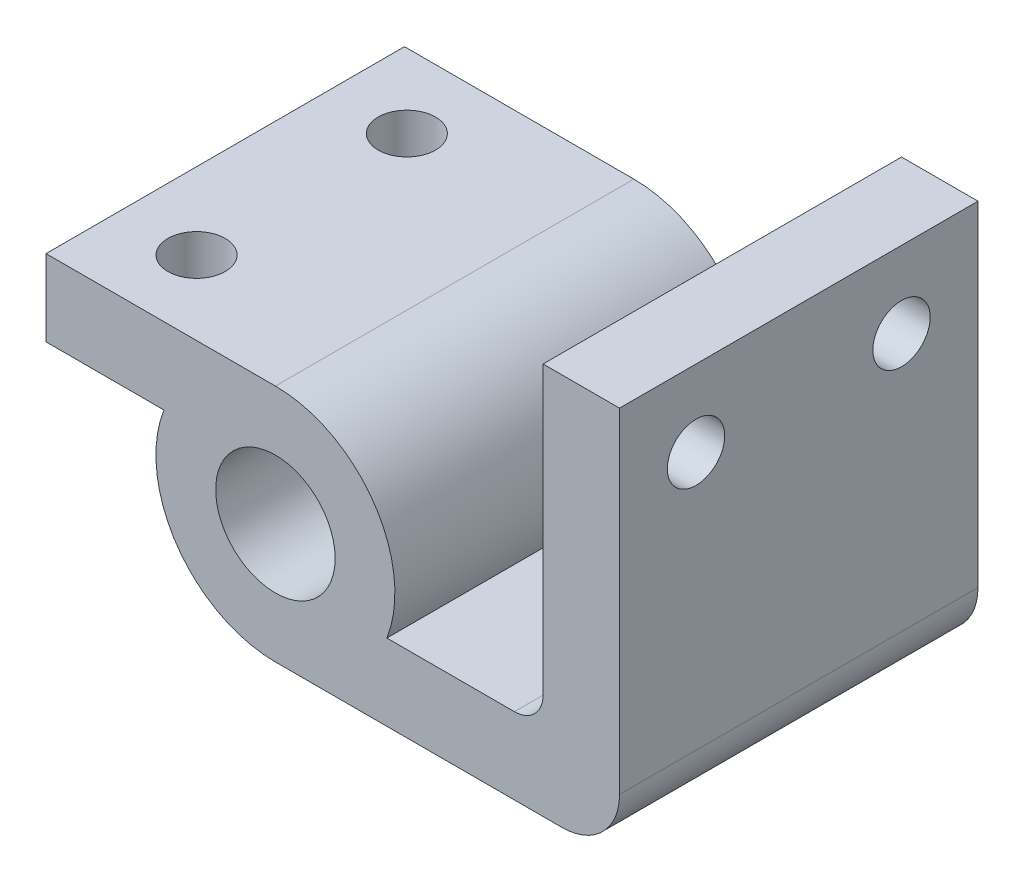
ISO-10303-21;
HEADER;
FILE_DESCRIPTION(('STEP AP214'),'2;1');
FILE_NAME('part.step','',(''),(''),'','','');
FILE_SCHEMA(('AUTOMOTIVE_DESIGN { 1 0 10303 214 1 1 1 1 }'));
ENDSEC;
DATA;
#1=APPLICATION_CONTEXT('core data for automotive mechanical design processes');
#2=APPLICATION_PROTOCOL_DEFINITION('international standard','automotive_design',2000,#1);
#3=PRODUCT_CONTEXT('',#1,'mechanical');
#4=PRODUCT('Part','Part','',(#3));
#5=PRODUCT_RELATED_PRODUCT_CATEGORY('part','',(#4));
#6=PRODUCT_DEFINITION_FORMATION('','',#4);
#7=PRODUCT_DEFINITION_CONTEXT('part definition',#1,'design');
#8=PRODUCT_DEFINITION('design','',#6,#7);
#9=PRODUCT_DEFINITION_SHAPE('','',#8);
#10=(LENGTH_UNIT() NAMED_UNIT(*) SI_UNIT(.MILLI.,.METRE.));
#11=(NAMED_UNIT(*) PLANE_ANGLE_UNIT() SI_UNIT($,.RADIAN.));
#12=(NAMED_UNIT(*) SI_UNIT($,.STERADIAN.) SOLID_ANGLE_UNIT());
#13=UNCERTAINTY_MEASURE_WITH_UNIT(LENGTH_MEASURE(1.E-05),#10,'distance_accuracy_value','');
#14=(GEOMETRIC_REPRESENTATION_CONTEXT(3) GLOBAL_UNCERTAINTY_ASSIGNED_CONTEXT((#13)) GLOBAL_UNIT_ASSIGNED_CONTEXT((#10,
#11,#12)) REPRESENTATION_CONTEXT('',''));
#15=CARTESIAN_POINT('',(0.,0.,0.));
#16=DIRECTION('',(0.,0.,1.));
#17=DIRECTION('',(1.,0.,0.));
#18=AXIS2_PLACEMENT_3D('',#15,#16,#17);
#19=CARTESIAN_POINT('',(0.,-25.,75.));
#20=DIRECTION('',(0.,1.,0.));
#21=DIRECTION('',(0.,0.,1.));
#22=AXIS2_PLACEMENT_3D('',#19,#20,#21);
#23=PLANE('',#22);
#24=DIRECTION('',(1.,0.,0.));
#25=VECTOR('',#24,1.);
#26=CARTESIAN_POINT('',(0.,-25.,0.));
#27=LINE('',#26,#25);
#28=CARTESIAN_POINT('',(0.,-25.,0.));
#29=VERTEX_POINT('',#28);
#30=CARTESIAN_POINT('',(59.9999999999999,-25.,0.));
#31=VERTEX_POINT('',#30);
#32=EDGE_CURVE('E166',#29,#31,#27,.T.);
#33=ORIENTED_EDGE('',*,*,#32,.T.);
#34=DIRECTION('',(0.,0.,-1.));
#35=VECTOR('',#34,1.);
#36=CARTESIAN_POINT('',(59.9999999999999,-25.,75.));
#37=LINE('',#36,#35);
#38=CARTESIAN_POINT('',(59.9999999999999,-25.,75.));
#39=VERTEX_POINT('',#38);
#40=EDGE_CURVE('E11',#39,#31,#37,.T.);
#41=ORIENTED_EDGE('',*,*,#40,.F.);
#42=DIRECTION('',(1.,0.,0.));
#43=VECTOR('',#42,1.);
#44=CARTESIAN_POINT('',(0.,-25.,75.));
#45=LINE('',#44,#43);
#46=CARTESIAN_POINT('',(0.,-25.,75.));
#47=VERTEX_POINT('',#46);
#48=EDGE_CURVE('E194',#47,#39,#45,.T.);
#49=ORIENTED_EDGE('',*,*,#48,.F.);
#50=DIRECTION('',(0.,0.,-1.));
#51=VECTOR('',#50,1.);
#52=CARTESIAN_POINT('',(0.,-25.,75.));
#53=LINE('',#52,#51);
#54=EDGE_CURVE('E164',#47,#29,#53,.T.);
#55=ORIENTED_EDGE('',*,*,#54,.T.);
#56=EDGE_LOOP('',(#33,#41,#49,#55));
#57=FACE_BOUND('',#56,.T.);
#58=ADVANCED_FACE('F50',(#57),#23,.F.);
#59=CARTESIAN_POINT('',(60.,-13.,75.));
#60=DIRECTION('',(0.,0.,-1.));
#61=DIRECTION('',(-1.,0.,0.));
#62=AXIS2_PLACEMENT_3D('',#59,#60,#61);
#63=CYLINDRICAL_SURFACE('',#62,12.);
#64=CARTESIAN_POINT('',(60.,-13.,0.));
#65=DIRECTION('',(0.,0.,1.));
#66=DIRECTION('',(1.,0.,0.));
#67=AXIS2_PLACEMENT_3D('',#64,#65,#66);
#68=CIRCLE('',#67,12.);
#69=CARTESIAN_POINT('',(72.,-12.9999999999999,0.));
#70=VERTEX_POINT('',#69);
#71=EDGE_CURVE('E175',#31,#70,#68,.T.);
#72=ORIENTED_EDGE('',*,*,#71,.T.);
#73=DIRECTION('',(0.,0.,-1.));
#74=VECTOR('',#73,1.);
#75=CARTESIAN_POINT('',(72.,-12.9999999999999,75.));
#76=LINE('',#75,#74);
#77=CARTESIAN_POINT('',(72.,-12.9999999999999,75.));
#78=VERTEX_POINT('',#77);
#79=EDGE_CURVE('E57',#78,#70,#76,.T.);
#80=ORIENTED_EDGE('',*,*,#79,.F.);
#81=CARTESIAN_POINT('',(60.,-13.,75.));
#82=DIRECTION('',(0.,0.,1.));
#83=DIRECTION('',(1.,0.,0.));
#84=AXIS2_PLACEMENT_3D('',#81,#82,#83);
#85=CIRCLE('',#84,12.);
#86=EDGE_CURVE('E117',#39,#78,#85,.T.);
#87=ORIENTED_EDGE('',*,*,#86,.F.);
#88=ORIENTED_EDGE('',*,*,#40,.T.);
#89=EDGE_LOOP('',(#72,#80,#87,#88));
#90=FACE_BOUND('',#89,.T.);
#91=ADVANCED_FACE('F286',(#90),#63,.T.);
#92=CARTESIAN_POINT('',(72.,0.,75.));
#93=DIRECTION('',(-1.,0.,0.));
#94=DIRECTION('',(0.,0.,1.));
#95=AXIS2_PLACEMENT_3D('',#92,#93,#94);
#96=PLANE('',#95);
#97=CARTESIAN_POINT('',(72.,41.,59.));
#98=DIRECTION('',(1.,0.,0.));
#99=DIRECTION('',(0.,0.,-1.));
#100=AXIS2_PLACEMENT_3D('',#97,#98,#99);
#101=CIRCLE('',#100,6.);
#102=CARTESIAN_POINT('',(72.,41.,53.));
#103=VERTEX_POINT('',#102);
#104=EDGE_CURVE('E224',#103,#103,#101,.T.);
#105=ORIENTED_EDGE('',*,*,#104,.F.);
#106=EDGE_LOOP('',(#105));
#107=FACE_BOUND('',#106,.T.);
#108=CARTESIAN_POINT('',(72.,41.,16.));
#109=DIRECTION('',(1.,0.,0.));
#110=DIRECTION('',(0.,0.,-1.));
#111=AXIS2_PLACEMENT_3D('',#108,#109,#110);
#112=CIRCLE('',#111,6.);
#113=CARTESIAN_POINT('',(72.,41.,10.));
#114=VERTEX_POINT('',#113);
#115=EDGE_CURVE('E229',#114,#114,#112,.T.);
#116=ORIENTED_EDGE('',*,*,#115,.F.);
#117=EDGE_LOOP('',(#116));
#118=FACE_BOUND('',#117,.T.);
#119=DIRECTION('',(0.,1.,0.));
#120=VECTOR('',#119,1.);
#121=CARTESIAN_POINT('',(72.,0.,0.));
#122=LINE('',#121,#120);
#123=CARTESIAN_POINT('',(72.,57.,0.));
#124=VERTEX_POINT('',#123);
#125=EDGE_CURVE('E172',#70,#124,#122,.T.);
#126=ORIENTED_EDGE('',*,*,#125,.T.);
#127=DIRECTION('',(0.,0.,-1.));
#128=VECTOR('',#127,1.);
#129=CARTESIAN_POINT('',(72.,57.,75.));
#130=LINE('',#129,#128);
#131=CARTESIAN_POINT('',(72.,57.,75.));
#132=VERTEX_POINT('',#131);
#133=EDGE_CURVE('E211',#132,#124,#130,.T.);
#134=ORIENTED_EDGE('',*,*,#133,.F.);
#135=DIRECTION('',(0.,1.,0.));
#136=VECTOR('',#135,1.);
#137=CARTESIAN_POINT('',(72.,0.,75.));
#138=LINE('',#137,#136);
#139=EDGE_CURVE('E247',#78,#132,#138,.T.);
#140=ORIENTED_EDGE('',*,*,#139,.F.);
#141=ORIENTED_EDGE('',*,*,#79,.T.);
#142=EDGE_LOOP('',(#126,#134,#140,#141));
#143=FACE_BOUND('',#142,.T.);
#144=ADVANCED_FACE('F293',(#107,#118,#143),#96,.F.);
#145=CARTESIAN_POINT('',(0.,57.,75.));
#146=DIRECTION('',(0.,-1.,0.));
#147=DIRECTION('',(0.,0.,-1.));
#148=AXIS2_PLACEMENT_3D('',#145,#146,#147);
#149=PLANE('',#148);
#150=DIRECTION('',(-1.,0.,0.));
#151=VECTOR('',#150,1.);
#152=CARTESIAN_POINT('',(0.,57.,0.));
#153=LINE('',#152,#151);
#154=CARTESIAN_POINT('',(56.,57.,0.));
#155=VERTEX_POINT('',#154);
#156=EDGE_CURVE('E180',#124,#155,#153,.T.);
#157=ORIENTED_EDGE('',*,*,#156,.T.);
#158=DIRECTION('',(0.,0.,-1.));
#159=VECTOR('',#158,1.);
#160=CARTESIAN_POINT('',(56.,57.,75.));
#161=LINE('',#160,#159);
#162=CARTESIAN_POINT('',(56.,57.,75.));
#163=VERTEX_POINT('',#162);
#164=EDGE_CURVE('E208',#163,#155,#161,.T.);
#165=ORIENTED_EDGE('',*,*,#164,.F.);
#166=DIRECTION('',(-1.,0.,0.));
#167=VECTOR('',#166,1.);
#168=CARTESIAN_POINT('',(0.,57.,75.));
#169=LINE('',#168,#167);
#170=EDGE_CURVE('E248',#132,#163,#169,.T.);
#171=ORIENTED_EDGE('',*,*,#170,.F.);
#172=ORIENTED_EDGE('',*,*,#133,.T.);
#173=EDGE_LOOP('',(#157,#165,#171,#172));
#174=FACE_BOUND('',#173,.T.);
#175=ADVANCED_FACE('F297',(#174),#149,.F.);
#176=CARTESIAN_POINT('',(56.,0.,75.));
#177=DIRECTION('',(1.,0.,0.));
#178=DIRECTION('',(0.,0.,-1.));
#179=AXIS2_PLACEMENT_3D('',#176,#177,#178);
#180=PLANE('',#179);
#181=CARTESIAN_POINT('',(56.,41.,59.));
#182=DIRECTION('',(1.,0.,0.));
#183=DIRECTION('',(0.,0.,-1.));
#184=AXIS2_PLACEMENT_3D('',#181,#182,#183);
#185=CIRCLE('',#184,6.);
#186=CARTESIAN_POINT('',(56.,41.,53.));
#187=VERTEX_POINT('',#186);
#188=EDGE_CURVE('E49',#187,#187,#185,.T.);
#189=ORIENTED_EDGE('',*,*,#188,.T.);
#190=EDGE_LOOP('',(#189));
#191=FACE_BOUND('',#190,.T.);
#192=CARTESIAN_POINT('',(56.,41.,16.));
#193=DIRECTION('',(1.,0.,0.));
#194=DIRECTION('',(0.,0.,-1.));
#195=AXIS2_PLACEMENT_3D('',#192,#193,#194);
#196=CIRCLE('',#195,6.);
#197=CARTESIAN_POINT('',(56.,41.,10.));
#198=VERTEX_POINT('',#197);
#199=EDGE_CURVE('E222',#198,#198,#196,.T.);
#200=ORIENTED_EDGE('',*,*,#199,.T.);
#201=EDGE_LOOP('',(#200));
#202=FACE_BOUND('',#201,.T.);
#203=DIRECTION('',(0.,-1.,0.));
#204=VECTOR('',#203,1.);
#205=CARTESIAN_POINT('',(56.,0.,0.));
#206=LINE('',#205,#204);
#207=CARTESIAN_POINT('',(56.,-2.99999999999996,0.));
#208=VERTEX_POINT('',#207);
#209=EDGE_CURVE('E179',#155,#208,#206,.T.);
#210=ORIENTED_EDGE('',*,*,#209,.T.);
#211=DIRECTION('',(0.,0.,-1.));
#212=VECTOR('',#211,1.);
#213=CARTESIAN_POINT('',(56.,-2.99999999999996,75.));
#214=LINE('',#213,#212);
#215=CARTESIAN_POINT('',(56.,-2.99999999999996,75.));
#216=VERTEX_POINT('',#215);
#217=EDGE_CURVE('E206',#216,#208,#214,.T.);
#218=ORIENTED_EDGE('',*,*,#217,.F.);
#219=DIRECTION('',(0.,-1.,0.));
#220=VECTOR('',#219,1.);
#221=CARTESIAN_POINT('',(56.,0.,75.));
#222=LINE('',#221,#220);
#223=EDGE_CURVE('E246',#163,#216,#222,.T.);
#224=ORIENTED_EDGE('',*,*,#223,.F.);
#225=ORIENTED_EDGE('',*,*,#164,.T.);
#226=EDGE_LOOP('',(#210,#218,#224,#225));
#227=FACE_BOUND('',#226,.T.);
#228=ADVANCED_FACE('F301',(#191,#202,#227),#180,.F.);
#229=CARTESIAN_POINT('',(50.,-3.,75.));
#230=DIRECTION('',(0.,0.,-1.));
#231=DIRECTION('',(-1.,0.,0.));
#232=AXIS2_PLACEMENT_3D('',#229,#230,#231);
#233=CYLINDRICAL_SURFACE('',#232,6.);
#234=CARTESIAN_POINT('',(50.,-3.,0.));
#235=DIRECTION('',(0.,0.,1.));
#236=DIRECTION('',(1.,0.,0.));
#237=AXIS2_PLACEMENT_3D('',#234,#235,#236);
#238=CIRCLE('',#237,6.);
#239=CARTESIAN_POINT('',(50.,-9.,0.));
#240=VERTEX_POINT('',#239);
#241=EDGE_CURVE('E185',#240,#208,#238,.T.);
#242=ORIENTED_EDGE('',*,*,#241,.F.);
#243=DIRECTION('',(0.,0.,-1.));
#244=VECTOR('',#243,1.);
#245=CARTESIAN_POINT('',(50.,-9.,75.));
#246=LINE('',#245,#244);
#247=CARTESIAN_POINT('',(50.,-9.,75.));
#248=VERTEX_POINT('',#247);
#249=EDGE_CURVE('E204',#248,#240,#246,.T.);
#250=ORIENTED_EDGE('',*,*,#249,.F.);
#251=CARTESIAN_POINT('',(50.,-3.,75.));
#252=DIRECTION('',(0.,0.,1.));
#253=DIRECTION('',(1.,0.,0.));
#254=AXIS2_PLACEMENT_3D('',#251,#252,#253);
#255=CIRCLE('',#254,6.);
#256=EDGE_CURVE('E252',#248,#216,#255,.T.);
#257=ORIENTED_EDGE('',*,*,#256,.T.);
#258=ORIENTED_EDGE('',*,*,#217,.T.);
#259=EDGE_LOOP('',(#242,#250,#257,#258));
#260=FACE_BOUND('',#259,.T.);
#261=ADVANCED_FACE('F310',(#260),#233,.F.);
#262=CARTESIAN_POINT('',(0.,-9.,75.));
#263=DIRECTION('',(0.,-1.,0.));
#264=DIRECTION('',(0.,0.,-1.));
#265=AXIS2_PLACEMENT_3D('',#262,#263,#264);
#266=PLANE('',#265);
#267=DIRECTION('',(-1.,0.,0.));
#268=VECTOR('',#267,1.);
#269=CARTESIAN_POINT('',(0.,-9.,0.));
#270=LINE('',#269,#268);
#271=CARTESIAN_POINT('',(23.3238075793812,-9.,0.));
#272=VERTEX_POINT('',#271);
#273=EDGE_CURVE('E183',#240,#272,#270,.T.);
#274=ORIENTED_EDGE('',*,*,#273,.T.);
#275=DIRECTION('',(0.,0.,-1.));
#276=VECTOR('',#275,1.);
#277=CARTESIAN_POINT('',(23.3238075793812,-9.,75.));
#278=LINE('',#277,#276);
#279=CARTESIAN_POINT('',(23.3238075793812,-9.,75.));
#280=VERTEX_POINT('',#279);
#281=EDGE_CURVE('E203',#280,#272,#278,.T.);
#282=ORIENTED_EDGE('',*,*,#281,.F.);
#283=DIRECTION('',(-1.,0.,0.));
#284=VECTOR('',#283,1.);
#285=CARTESIAN_POINT('',(0.,-9.,75.));
#286=LINE('',#285,#284);
#287=EDGE_CURVE('E254',#248,#280,#286,.T.);
#288=ORIENTED_EDGE('',*,*,#287,.F.);
#289=ORIENTED_EDGE('',*,*,#249,.T.);
#290=EDGE_LOOP('',(#274,#282,#288,#289));
#291=FACE_BOUND('',#290,.T.);
#292=ADVANCED_FACE('F311',(#291),#266,.F.);
#293=CARTESIAN_POINT('',(0.,0.,75.));
#294=DIRECTION('',(0.,0.,-1.));
#295=DIRECTION('',(-1.,0.,0.));
#296=AXIS2_PLACEMENT_3D('',#293,#294,#295);
#297=CYLINDRICAL_SURFACE('',#296,25.);
#298=CARTESIAN_POINT('',(0.,0.,0.));
#299=DIRECTION('',(0.,0.,1.));
#300=DIRECTION('',(1.,0.,0.));
#301=AXIS2_PLACEMENT_3D('',#298,#299,#300);
#302=CIRCLE('',#301,25.);
#303=CARTESIAN_POINT('',(0.,25.,0.));
#304=VERTEX_POINT('',#303);
#305=EDGE_CURVE('E190',#272,#304,#302,.T.);
#306=ORIENTED_EDGE('',*,*,#305,.T.);
#307=DIRECTION('',(0.,0.,-1.));
#308=VECTOR('',#307,1.);
#309=CARTESIAN_POINT('',(0.,25.,75.));
#310=LINE('',#309,#308);
#311=CARTESIAN_POINT('',(0.,25.,75.));
#312=VERTEX_POINT('',#311);
#313=EDGE_CURVE('E196',#312,#304,#310,.T.);
#314=ORIENTED_EDGE('',*,*,#313,.F.);
#315=CARTESIAN_POINT('',(0.,0.,75.));
#316=DIRECTION('',(0.,0.,1.));
#317=DIRECTION('',(1.,0.,0.));
#318=AXIS2_PLACEMENT_3D('',#315,#316,#317);
#319=CIRCLE('',#318,25.);
#320=EDGE_CURVE('E260',#280,#312,#319,.T.);
#321=ORIENTED_EDGE('',*,*,#320,.F.);
#322=ORIENTED_EDGE('',*,*,#281,.T.);
#323=EDGE_LOOP('',(#306,#314,#321,#322));
#324=FACE_BOUND('',#323,.T.);
#325=ADVANCED_FACE('F262',(#324),#297,.T.);
#326=CARTESIAN_POINT('',(0.,25.,75.));
#327=DIRECTION('',(0.,-1.,0.));
#328=DIRECTION('',(0.,0.,-1.));
#329=AXIS2_PLACEMENT_3D('',#326,#327,#328);
#330=PLANE('',#329);
#331=CARTESIAN_POINT('',(-32.,25.,15.5));
#332=DIRECTION('',(0.,1.,0.));
#333=DIRECTION('',(0.,0.,1.));
#334=AXIS2_PLACEMENT_3D('',#331,#332,#333);
#335=CIRCLE('',#334,6.);
#336=CARTESIAN_POINT('',(-32.,25.,21.5));
#337=VERTEX_POINT('',#336);
#338=EDGE_CURVE('E218',#337,#337,#335,.T.);
#339=ORIENTED_EDGE('',*,*,#338,.F.);
#340=EDGE_LOOP('',(#339));
#341=FACE_BOUND('',#340,.T.);
#342=CARTESIAN_POINT('',(-32.,25.,59.5));
#343=DIRECTION('',(0.,1.,0.));
#344=DIRECTION('',(0.,0.,1.));
#345=AXIS2_PLACEMENT_3D('',#342,#343,#344);
#346=CIRCLE('',#345,6.);
#347=CARTESIAN_POINT('',(-32.,25.,65.5));
#348=VERTEX_POINT('',#347);
#349=EDGE_CURVE('E230',#348,#348,#346,.T.);
#350=ORIENTED_EDGE('',*,*,#349,.F.);
#351=EDGE_LOOP('',(#350));
#352=FACE_BOUND('',#351,.T.);
#353=DIRECTION('',(-1.,0.,0.));
#354=VECTOR('',#353,1.);
#355=CARTESIAN_POINT('',(0.,25.,0.));
#356=LINE('',#355,#354);
#357=CARTESIAN_POINT('',(-48.,25.,0.));
#358=VERTEX_POINT('',#357);
#359=EDGE_CURVE('E189',#304,#358,#356,.T.);
#360=ORIENTED_EDGE('',*,*,#359,.T.);
#361=DIRECTION('',(0.,0.,-1.));
#362=VECTOR('',#361,1.);
#363=CARTESIAN_POINT('',(-48.,25.,75.));
#364=LINE('',#363,#362);
#365=CARTESIAN_POINT('',(-48.,25.,75.));
#366=VERTEX_POINT('',#365);
#367=EDGE_CURVE('E159',#366,#358,#364,.T.);
#368=ORIENTED_EDGE('',*,*,#367,.F.);
#369=DIRECTION('',(-1.,0.,0.));
#370=VECTOR('',#369,1.);
#371=CARTESIAN_POINT('',(0.,25.,75.));
#372=LINE('',#371,#370);
#373=EDGE_CURVE('E151',#312,#366,#372,.T.);
#374=ORIENTED_EDGE('',*,*,#373,.F.);
#375=ORIENTED_EDGE('',*,*,#313,.T.);
#376=EDGE_LOOP('',(#360,#368,#374,#375));
#377=FACE_BOUND('',#376,.T.);
#378=ADVANCED_FACE('F268',(#341,#352,#377),#330,.F.);
#379=CARTESIAN_POINT('',(-48.,0.,75.));
#380=DIRECTION('',(1.,0.,0.));
#381=DIRECTION('',(0.,0.,-1.));
#382=AXIS2_PLACEMENT_3D('',#379,#380,#381);
#383=PLANE('',#382);
#384=DIRECTION('',(0.,-1.,0.));
#385=VECTOR('',#384,1.);
#386=CARTESIAN_POINT('',(-48.,0.,0.));
#387=LINE('',#386,#385);
#388=CARTESIAN_POINT('',(-48.,9.,0.));
#389=VERTEX_POINT('',#388);
#390=EDGE_CURVE('E157',#358,#389,#387,.T.);
#391=ORIENTED_EDGE('',*,*,#390,.T.);
#392=DIRECTION('',(0.,0.,-1.));
#393=VECTOR('',#392,1.);
#394=CARTESIAN_POINT('',(-48.,9.,75.));
#395=LINE('',#394,#393);
#396=CARTESIAN_POINT('',(-48.,9.,75.));
#397=VERTEX_POINT('',#396);
#398=EDGE_CURVE('E156',#397,#389,#395,.T.);
#399=ORIENTED_EDGE('',*,*,#398,.F.);
#400=DIRECTION('',(0.,-1.,0.));
#401=VECTOR('',#400,1.);
#402=CARTESIAN_POINT('',(-48.,0.,75.));
#403=LINE('',#402,#401);
#404=EDGE_CURVE('E144',#366,#397,#403,.T.);
#405=ORIENTED_EDGE('',*,*,#404,.F.);
#406=ORIENTED_EDGE('',*,*,#367,.T.);
#407=EDGE_LOOP('',(#391,#399,#405,#406));
#408=FACE_BOUND('',#407,.T.);
#409=ADVANCED_FACE('F160',(#408),#383,.F.);
#410=CARTESIAN_POINT('',(0.,9.,75.));
#411=DIRECTION('',(0.,1.,0.));
#412=DIRECTION('',(0.,0.,1.));
#413=AXIS2_PLACEMENT_3D('',#410,#411,#412);
#414=PLANE('',#413);
#415=CARTESIAN_POINT('',(-32.,9.,15.5));
#416=DIRECTION('',(0.,1.,0.));
#417=DIRECTION('',(0.,0.,1.));
#418=AXIS2_PLACEMENT_3D('',#415,#416,#417);
#419=CIRCLE('',#418,6.);
#420=CARTESIAN_POINT('',(-32.,9.,21.5));
#421=VERTEX_POINT('',#420);
#422=EDGE_CURVE('E171',#421,#421,#419,.T.);
#423=ORIENTED_EDGE('',*,*,#422,.T.);
#424=EDGE_LOOP('',(#423));
#425=FACE_BOUND('',#424,.T.);
#426=CARTESIAN_POINT('',(-32.,9.,59.5));
#427=DIRECTION('',(0.,1.,0.));
#428=DIRECTION('',(0.,0.,1.));
#429=AXIS2_PLACEMENT_3D('',#426,#427,#428);
#430=CIRCLE('',#429,6.);
#431=CARTESIAN_POINT('',(-32.,9.,65.5));
#432=VERTEX_POINT('',#431);
#433=EDGE_CURVE('E216',#432,#432,#430,.T.);
#434=ORIENTED_EDGE('',*,*,#433,.T.);
#435=EDGE_LOOP('',(#434));
#436=FACE_BOUND('',#435,.T.);
#437=DIRECTION('',(1.,0.,0.));
#438=VECTOR('',#437,1.);
#439=CARTESIAN_POINT('',(0.,9.,0.));
#440=LINE('',#439,#438);
#441=CARTESIAN_POINT('',(-23.3238075793812,9.,0.));
#442=VERTEX_POINT('',#441);
#443=EDGE_CURVE('E106',#389,#442,#440,.T.);
#444=ORIENTED_EDGE('',*,*,#443,.T.);
#445=DIRECTION('',(0.,0.,-1.));
#446=VECTOR('',#445,1.);
#447=CARTESIAN_POINT('',(-23.3238075793812,9.,75.));
#448=LINE('',#447,#446);
#449=CARTESIAN_POINT('',(-23.3238075793812,9.,75.));
#450=VERTEX_POINT('',#449);
#451=EDGE_CURVE('E161',#450,#442,#448,.T.);
#452=ORIENTED_EDGE('',*,*,#451,.F.);
#453=DIRECTION('',(1.,0.,0.));
#454=VECTOR('',#453,1.);
#455=CARTESIAN_POINT('',(0.,9.,75.));
#456=LINE('',#455,#454);
#457=EDGE_CURVE('E149',#397,#450,#456,.T.);
#458=ORIENTED_EDGE('',*,*,#457,.F.);
#459=ORIENTED_EDGE('',*,*,#398,.T.);
#460=EDGE_LOOP('',(#444,#452,#458,#459));
#461=FACE_BOUND('',#460,.T.);
#462=ADVANCED_FACE('F162',(#425,#436,#461),#414,.F.);
#463=CARTESIAN_POINT('',(0.,0.,75.));
#464=DIRECTION('',(0.,0.,-1.));
#465=DIRECTION('',(-1.,0.,0.));
#466=AXIS2_PLACEMENT_3D('',#463,#464,#465);
#467=CYLINDRICAL_SURFACE('',#466,25.);
#468=CARTESIAN_POINT('',(0.,0.,0.));
#469=DIRECTION('',(0.,0.,1.));
#470=DIRECTION('',(1.,0.,0.));
#471=AXIS2_PLACEMENT_3D('',#468,#469,#470);
#472=CIRCLE('',#471,25.);
#473=EDGE_CURVE('E115',#442,#29,#472,.T.);
#474=ORIENTED_EDGE('',*,*,#473,.T.);
#475=ORIENTED_EDGE('',*,*,#54,.F.);
#476=CARTESIAN_POINT('',(0.,0.,75.));
#477=DIRECTION('',(0.,0.,1.));
#478=DIRECTION('',(1.,0.,0.));
#479=AXIS2_PLACEMENT_3D('',#476,#477,#478);
#480=CIRCLE('',#479,25.);
#481=EDGE_CURVE('E62',#450,#47,#480,.T.);
#482=ORIENTED_EDGE('',*,*,#481,.F.);
#483=ORIENTED_EDGE('',*,*,#451,.T.);
#484=EDGE_LOOP('',(#474,#475,#482,#483));
#485=FACE_BOUND('',#484,.T.);
#486=ADVANCED_FACE('F277',(#485),#467,.T.);
#487=CARTESIAN_POINT('',(0.,0.,75.));
#488=DIRECTION('',(0.,0.,1.));
#489=DIRECTION('',(1.,0.,0.));
#490=AXIS2_PLACEMENT_3D('',#487,#488,#489);
#491=PLANE('',#490);
#492=CARTESIAN_POINT('',(0.,0.,75.));
#493=DIRECTION('',(0.,0.,1.));
#494=DIRECTION('',(1.,0.,0.));
#495=AXIS2_PLACEMENT_3D('',#492,#493,#494);
#496=CIRCLE('',#495,12.5);
#497=CARTESIAN_POINT('',(12.5,0.,75.));
#498=VERTEX_POINT('',#497);
#499=EDGE_CURVE('E240',#498,#498,#496,.T.);
#500=ORIENTED_EDGE('',*,*,#499,.F.);
#501=EDGE_LOOP('',(#500));
#502=FACE_BOUND('',#501,.T.);
#503=ORIENTED_EDGE('',*,*,#48,.T.);
#504=ORIENTED_EDGE('',*,*,#86,.T.);
#505=ORIENTED_EDGE('',*,*,#139,.T.);
#506=ORIENTED_EDGE('',*,*,#170,.T.);
#507=ORIENTED_EDGE('',*,*,#223,.T.);
#508=ORIENTED_EDGE('',*,*,#256,.F.);
#509=ORIENTED_EDGE('',*,*,#287,.T.);
#510=ORIENTED_EDGE('',*,*,#320,.T.);
#511=ORIENTED_EDGE('',*,*,#373,.T.);
#512=ORIENTED_EDGE('',*,*,#404,.T.);
#513=ORIENTED_EDGE('',*,*,#457,.T.);
#514=ORIENTED_EDGE('',*,*,#481,.T.);
#515=EDGE_LOOP('',(#503,#504,#505,#506,#507,#508,#509,#510,#511,#512,#513,#514));
#516=FACE_BOUND('',#515,.T.);
#517=ADVANCED_FACE('F150',(#502,#516),#491,.T.);
#518=CARTESIAN_POINT('',(0.,0.,0.));
#519=DIRECTION('',(0.,0.,1.));
#520=DIRECTION('',(1.,0.,0.));
#521=AXIS2_PLACEMENT_3D('',#518,#519,#520);
#522=PLANE('',#521);
#523=CARTESIAN_POINT('',(0.,0.,0.));
#524=DIRECTION('',(0.,0.,1.));
#525=DIRECTION('',(1.,0.,0.));
#526=AXIS2_PLACEMENT_3D('',#523,#524,#525);
#527=CIRCLE('',#526,12.5);
#528=CARTESIAN_POINT('',(12.5,0.,0.));
#529=VERTEX_POINT('',#528);
#530=EDGE_CURVE('E234',#529,#529,#527,.T.);
#531=ORIENTED_EDGE('',*,*,#530,.T.);
#532=EDGE_LOOP('',(#531));
#533=FACE_BOUND('',#532,.T.);
#534=ORIENTED_EDGE('',*,*,#32,.F.);
#535=ORIENTED_EDGE('',*,*,#473,.F.);
#536=ORIENTED_EDGE('',*,*,#443,.F.);
#537=ORIENTED_EDGE('',*,*,#390,.F.);
#538=ORIENTED_EDGE('',*,*,#359,.F.);
#539=ORIENTED_EDGE('',*,*,#305,.F.);
#540=ORIENTED_EDGE('',*,*,#273,.F.);
#541=ORIENTED_EDGE('',*,*,#241,.T.);
#542=ORIENTED_EDGE('',*,*,#209,.F.);
#543=ORIENTED_EDGE('',*,*,#156,.F.);
#544=ORIENTED_EDGE('',*,*,#125,.F.);
#545=ORIENTED_EDGE('',*,*,#71,.F.);
#546=EDGE_LOOP('',(#534,#535,#536,#537,#538,#539,#540,#541,#542,#543,#544,#545));
#547=FACE_BOUND('',#546,.T.);
#548=ADVANCED_FACE('F271',(#533,#547),#522,.F.);
#549=CARTESIAN_POINT('',(-32.,-50.,59.5));
#550=DIRECTION('',(0.,1.,0.));
#551=DIRECTION('',(0.,0.,1.));
#552=AXIS2_PLACEMENT_3D('',#549,#550,#551);
#553=CYLINDRICAL_SURFACE('',#552,6.);
#554=ORIENTED_EDGE('',*,*,#349,.T.);
#555=EDGE_LOOP('',(#554));
#556=FACE_BOUND('',#555,.T.);
#557=ORIENTED_EDGE('',*,*,#433,.F.);
#558=EDGE_LOOP('',(#557));
#559=FACE_BOUND('',#558,.T.);
#560=ADVANCED_FACE('F414',(#556,#559),#553,.F.);
#561=CARTESIAN_POINT('',(-32.,-50.,15.5));
#562=DIRECTION('',(0.,1.,0.));
#563=DIRECTION('',(0.,0.,1.));
#564=AXIS2_PLACEMENT_3D('',#561,#562,#563);
#565=CYLINDRICAL_SURFACE('',#564,6.);
#566=ORIENTED_EDGE('',*,*,#338,.T.);
#567=EDGE_LOOP('',(#566));
#568=FACE_BOUND('',#567,.T.);
#569=ORIENTED_EDGE('',*,*,#422,.F.);
#570=EDGE_LOOP('',(#569));
#571=FACE_BOUND('',#570,.T.);
#572=ADVANCED_FACE('F419',(#568,#571),#565,.F.);
#573=CARTESIAN_POINT('',(-3.,41.,16.));
#574=DIRECTION('',(1.,0.,0.));
#575=DIRECTION('',(0.,0.,-1.));
#576=AXIS2_PLACEMENT_3D('',#573,#574,#575);
#577=CYLINDRICAL_SURFACE('',#576,6.);
#578=ORIENTED_EDGE('',*,*,#115,.T.);
#579=EDGE_LOOP('',(#578));
#580=FACE_BOUND('',#579,.T.);
#581=ORIENTED_EDGE('',*,*,#199,.F.);
#582=EDGE_LOOP('',(#581));
#583=FACE_BOUND('',#582,.T.);
#584=ADVANCED_FACE('F433',(#580,#583),#577,.F.);
#585=CARTESIAN_POINT('',(-3.,41.,59.));
#586=DIRECTION('',(1.,0.,0.));
#587=DIRECTION('',(0.,0.,-1.));
#588=AXIS2_PLACEMENT_3D('',#585,#586,#587);
#589=CYLINDRICAL_SURFACE('',#588,6.);
#590=ORIENTED_EDGE('',*,*,#104,.T.);
#591=EDGE_LOOP('',(#590));
#592=FACE_BOUND('',#591,.T.);
#593=ORIENTED_EDGE('',*,*,#188,.F.);
#594=EDGE_LOOP('',(#593));
#595=FACE_BOUND('',#594,.T.);
#596=ADVANCED_FACE('F451',(#592,#595),#589,.F.);
#597=CARTESIAN_POINT('',(0.,0.,0.));
#598=DIRECTION('',(0.,0.,1.));
#599=DIRECTION('',(1.,0.,0.));
#600=AXIS2_PLACEMENT_3D('',#597,#598,#599);
#601=CYLINDRICAL_SURFACE('',#600,12.5);
#602=ORIENTED_EDGE('',*,*,#530,.F.);
#603=EDGE_LOOP('',(#602));
#604=FACE_BOUND('',#603,.T.);
#605=ORIENTED_EDGE('',*,*,#499,.T.);
#606=EDGE_LOOP('',(#605));
#607=FACE_BOUND('',#606,.T.);
#608=ADVANCED_FACE('F470',(#604,#607),#601,.F.);
#609=CLOSED_SHELL('',(#58,#91,#144,#175,#228,#261,#292,#325,#378,#409,#462,#486,#517,#548,#560,
#572,#584,#596,#608));
#610=MANIFOLD_SOLID_BREP('B2',#609);
#611=ADVANCED_BREP_SHAPE_REPRESENTATION('',(#18,#610),#14);
#612=SHAPE_DEFINITION_REPRESENTATION(#9,#611);
ENDSEC;
END-ISO-10303-21;
